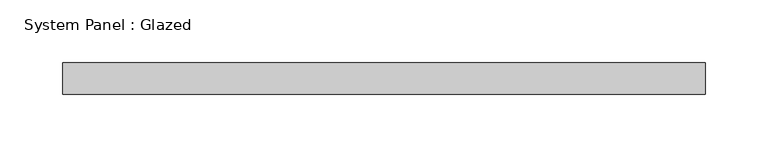
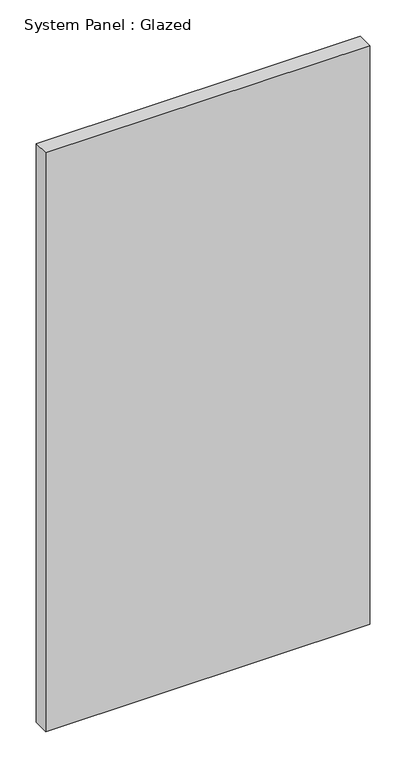
"""IFC4 building model written with IfcOpenShell, lengths in millimetres: plate geometry, System Panel : Glazed."""

from ifc_helpers import new_model, si_unit, origin, origin_with_axes, place, context, project, spatial, polyline, outline, extrude, source, transform, mapped, element, save


def system_panel_glazed_4cc38c21(model_context):
    return source(origin(), model_context, "Body", "SweptSolid", [
        extrude(outline(polyline([(257.175, 19.05), (-257.175, 19.05), (-257.175, 44.45), (257.175, 44.45), (257.175, 19.05)])), origin_with_axes(), (0.0, 0.0, 1.0), 971.55),
    ])


if __name__ == "__main__":
    model = new_model("IFC4")
    model_context = context("Model", 3, world=origin())
    ifc_project = project(units=[si_unit("LENGTHUNIT", "METRE", prefix="MILLI")], contexts=[model_context])
    site = spatial("IfcSite", under=ifc_project)
    building = spatial("IfcBuilding", under=site)
    placement = place(None, origin())
    system_panel_glazed_shape = system_panel_glazed_4cc38c21(model_context)
    element("IfcPlate", 1, ObjectType="System Panel : Glazed", at=placement, inside=building, context=model_context, shape_type="MappedRepresentation", body=[
        mapped(system_panel_glazed_shape, transform((0.0, 0.0, 0.0), x_axis=(1.0, 0.0, 0.0), y_axis=(0.0, 1.0, 0.0), z_axis=(0.0, 0.0, 1.0))),
    ])
    save(model, "model.ifc")

# Revit data of these elements
# Type "System Panel : Glazed"
#   Construction Type Id = "GSP4R"
#   Analytic Construction = "1/8 in Pilkington single glazing"
#   Visual Light Transmittance = 0.9
#   Solar Heat Gain Coefficient = 0.86
#   Heat Transfer Coefficient (U) = 1.18115 BTU/(h·ft²·°F)
#   Define Thermal Properties by = 1
# Element 1 (IfcPlate, "System Panel : Glazed")
#   Materials on its faces: "Glass"
# Materials
#   "Glass": class "Glass", colour RGB 0 128 192, transparency 0.75, Description = "Soda Lime Glass", Cost = 0
